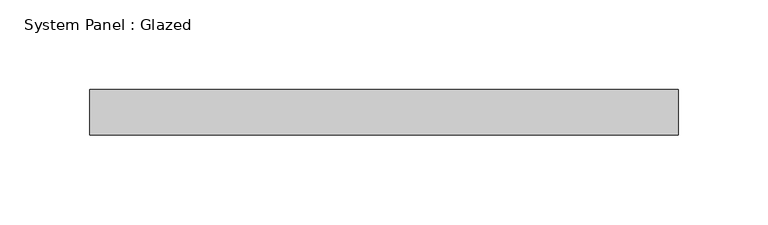
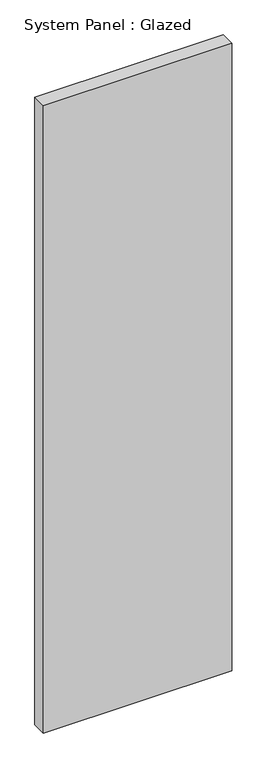
"""IFC4 building model written with IfcOpenShell, lengths in millimetres: plate geometry, System Panel : Glazed."""

from ifc_helpers import new_model, si_unit, origin, origin_with_axes, place, context, project, spatial, polyline, outline, extrude, source, transform, mapped, element, save


def system_panel_glazed_710bc1bd(model_context):
    return source(origin(), model_context, "Body", "SweptSolid", [
        extrude(outline(polyline([(164.277455, 19.05), (-164.277455, 19.05), (-164.277455, 44.45), (164.277455, 44.45), (164.277455, 19.05)])), origin_with_axes(), (0.0, 0.0, 1.0), 1155.7),
    ])


if __name__ == "__main__":
    model = new_model("IFC4")
    model_context = context("Model", 3, world=origin())
    ifc_project = project(units=[si_unit("LENGTHUNIT", "METRE", prefix="MILLI")], contexts=[model_context])
    site = spatial("IfcSite", under=ifc_project)
    building = spatial("IfcBuilding", under=site)
    placement = place(None, origin())
    system_panel_glazed_shape = system_panel_glazed_710bc1bd(model_context)
    element("IfcPlate", 1, ObjectType="System Panel : Glazed", at=placement, inside=building, context=model_context, shape_type="MappedRepresentation", body=[
        mapped(system_panel_glazed_shape, transform((0.0, 0.0, 0.0), x_axis=(1.0, 0.0, 0.0), y_axis=(0.0, 1.0, 0.0), z_axis=(0.0, 0.0, 1.0))),
    ])
    save(model, "model.ifc")

# Revit data of these elements
# Type "System Panel : Glazed"
#   Construction Type Id = "GSP4R"
#   Analytic Construction = "1/8 in Pilkington single glazing"
#   Visual Light Transmittance = 0.9
#   Solar Heat Gain Coefficient = 0.86
#   Heat Transfer Coefficient (U) = 1.18115 BTU/(h·ft²·°F)
# Element 1 (IfcPlate, "System Panel : Glazed")
#   Materials on its faces: "Glass"
# Materials
#   "Glass": class "Glass", colour RGB 0 128 192, transparency 0.75, Description = "Soda Lime Glass", Cost = 0
